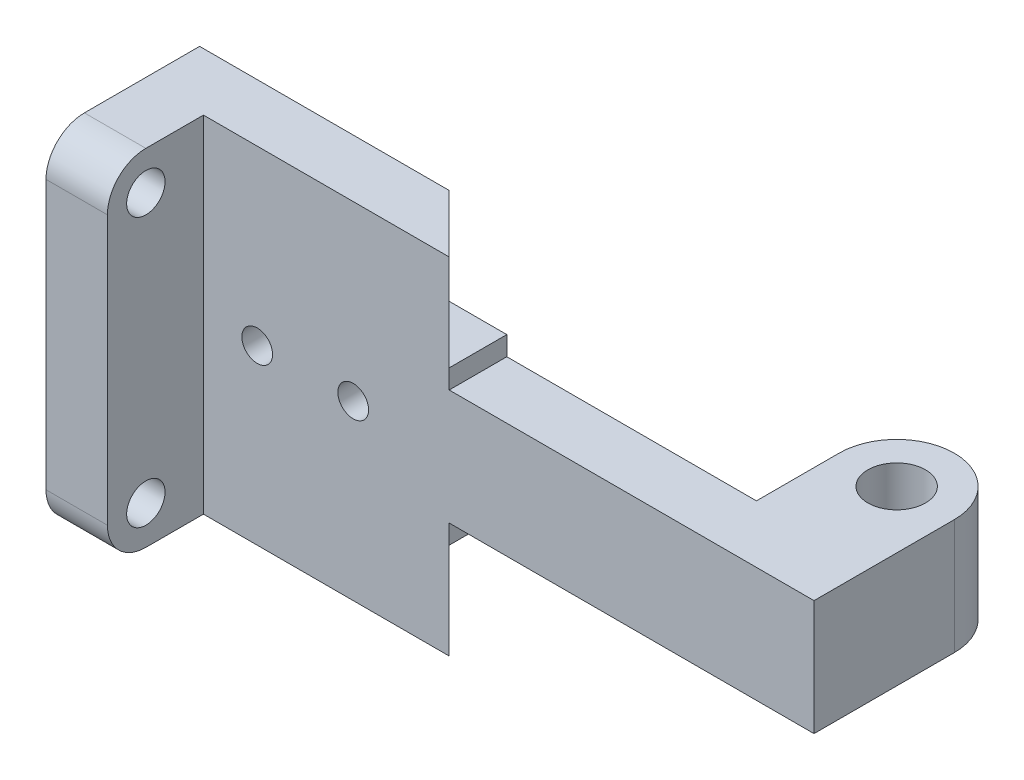
ISO-10303-21;
HEADER;
FILE_DESCRIPTION(('STEP AP214'),'2;1');
FILE_NAME('part.step','',(''),(''),'','','');
FILE_SCHEMA(('AUTOMOTIVE_DESIGN { 1 0 10303 214 1 1 1 1 }'));
ENDSEC;
DATA;
#1=APPLICATION_CONTEXT('core data for automotive mechanical design processes');
#2=APPLICATION_PROTOCOL_DEFINITION('international standard','automotive_design',2000,#1);
#3=PRODUCT_CONTEXT('',#1,'mechanical');
#4=PRODUCT('Part','Part','',(#3));
#5=PRODUCT_RELATED_PRODUCT_CATEGORY('part','',(#4));
#6=PRODUCT_DEFINITION_FORMATION('','',#4);
#7=PRODUCT_DEFINITION_CONTEXT('part definition',#1,'design');
#8=PRODUCT_DEFINITION('design','',#6,#7);
#9=PRODUCT_DEFINITION_SHAPE('','',#8);
#10=(LENGTH_UNIT() NAMED_UNIT(*) SI_UNIT(.MILLI.,.METRE.));
#11=(NAMED_UNIT(*) PLANE_ANGLE_UNIT() SI_UNIT($,.RADIAN.));
#12=(NAMED_UNIT(*) SI_UNIT($,.STERADIAN.) SOLID_ANGLE_UNIT());
#13=UNCERTAINTY_MEASURE_WITH_UNIT(LENGTH_MEASURE(1.E-05),#10,'distance_accuracy_value','');
#14=(GEOMETRIC_REPRESENTATION_CONTEXT(3) GLOBAL_UNCERTAINTY_ASSIGNED_CONTEXT((#13)) GLOBAL_UNIT_ASSIGNED_CONTEXT((#10,
#11,#12)) REPRESENTATION_CONTEXT('',''));
#15=CARTESIAN_POINT('',(0.,0.,0.));
#16=DIRECTION('',(0.,0.,1.));
#17=DIRECTION('',(1.,0.,0.));
#18=AXIS2_PLACEMENT_3D('',#15,#16,#17);
#19=CARTESIAN_POINT('',(-40.,90.,-7.5));
#20=DIRECTION('',(1.,0.,0.));
#21=DIRECTION('',(0.,0.,-1.));
#22=AXIS2_PLACEMENT_3D('',#19,#20,#21);
#23=PLANE('',#22);
#24=DIRECTION('',(0.,0.,1.));
#25=VECTOR('',#24,1.);
#26=CARTESIAN_POINT('',(-40.,0.,-7.5));
#27=LINE('',#26,#25);
#28=CARTESIAN_POINT('',(-40.,0.,-7.5));
#29=VERTEX_POINT('',#28);
#30=CARTESIAN_POINT('',(-40.,0.,22.5));
#31=VERTEX_POINT('',#30);
#32=EDGE_CURVE('E267',#29,#31,#27,.T.);
#33=ORIENTED_EDGE('',*,*,#32,.T.);
#34=CARTESIAN_POINT('',(-40.,9.99999999999999,22.5));
#35=DIRECTION('',(1.,0.,0.));
#36=DIRECTION('',(0.,0.,-1.));
#37=AXIS2_PLACEMENT_3D('',#34,#35,#36);
#38=CIRCLE('',#37,10.);
#39=CARTESIAN_POINT('',(-40.,10.,32.5));
#40=VERTEX_POINT('',#39);
#41=EDGE_CURVE('E48',#31,#40,#38,.F.);
#42=ORIENTED_EDGE('',*,*,#41,.T.);
#43=DIRECTION('',(0.,-1.,0.));
#44=VECTOR('',#43,1.);
#45=CARTESIAN_POINT('',(-40.,90.,32.5));
#46=LINE('',#45,#44);
#47=CARTESIAN_POINT('',(-40.,80.,32.5));
#48=VERTEX_POINT('',#47);
#49=EDGE_CURVE('E279',#48,#40,#46,.T.);
#50=ORIENTED_EDGE('',*,*,#49,.F.);
#51=CARTESIAN_POINT('',(-40.,80.,22.5));
#52=DIRECTION('',(1.,0.,0.));
#53=DIRECTION('',(0.,0.,-1.));
#54=AXIS2_PLACEMENT_3D('',#51,#52,#53);
#55=CIRCLE('',#54,10.);
#56=CARTESIAN_POINT('',(-40.,90.,22.5));
#57=VERTEX_POINT('',#56);
#58=EDGE_CURVE('E57',#48,#57,#55,.F.);
#59=ORIENTED_EDGE('',*,*,#58,.T.);
#60=DIRECTION('',(0.,0.,1.));
#61=VECTOR('',#60,1.);
#62=CARTESIAN_POINT('',(-40.,90.,-7.5));
#63=LINE('',#62,#61);
#64=CARTESIAN_POINT('',(-40.,90.,-7.5));
#65=VERTEX_POINT('',#64);
#66=EDGE_CURVE('E259',#65,#57,#63,.T.);
#67=ORIENTED_EDGE('',*,*,#66,.F.);
#68=DIRECTION('',(0.,-1.,0.));
#69=VECTOR('',#68,1.);
#70=CARTESIAN_POINT('',(-40.,90.,-7.5));
#71=LINE('',#70,#69);
#72=EDGE_CURVE('E283',#65,#29,#71,.T.);
#73=ORIENTED_EDGE('',*,*,#72,.T.);
#74=EDGE_LOOP('',(#33,#42,#50,#59,#67,#73));
#75=FACE_BOUND('',#74,.T.);
#76=CARTESIAN_POINT('',(-40.000012,9.99999999999999,22.5));
#77=DIRECTION('',(-1.,0.,0.));
#78=DIRECTION('',(0.,0.,1.));
#79=AXIS2_PLACEMENT_3D('',#76,#77,#78);
#80=CIRCLE('',#79,5.);
#81=CARTESIAN_POINT('',(-40.000012,9.99999999999999,27.5));
#82=VERTEX_POINT('',#81);
#83=EDGE_CURVE('E309',#82,#82,#80,.T.);
#84=ORIENTED_EDGE('',*,*,#83,.F.);
#85=EDGE_LOOP('',(#84));
#86=FACE_BOUND('',#85,.T.);
#87=CARTESIAN_POINT('',(-40.000012,80.,22.5));
#88=DIRECTION('',(-1.,0.,0.));
#89=DIRECTION('',(0.,0.,1.));
#90=AXIS2_PLACEMENT_3D('',#87,#88,#89);
#91=CIRCLE('',#90,5.);
#92=CARTESIAN_POINT('',(-40.000012,80.,27.5));
#93=VERTEX_POINT('',#92);
#94=EDGE_CURVE('E303',#93,#93,#91,.T.);
#95=ORIENTED_EDGE('',*,*,#94,.F.);
#96=EDGE_LOOP('',(#95));
#97=FACE_BOUND('',#96,.T.);
#98=ADVANCED_FACE('F39',(#75,#86,#97),#23,.F.);
#99=CARTESIAN_POINT('',(40.,90.,-7.5));
#100=DIRECTION('',(-1.,0.,0.));
#101=DIRECTION('',(0.,0.,1.));
#102=AXIS2_PLACEMENT_3D('',#99,#100,#101);
#103=PLANE('',#102);
#104=DIRECTION('',(0.,0.,1.));
#105=VECTOR('',#104,1.);
#106=CARTESIAN_POINT('',(40.,60.,7.5));
#107=LINE('',#106,#105);
#108=CARTESIAN_POINT('',(40.,60.,-7.5));
#109=VERTEX_POINT('',#108);
#110=CARTESIAN_POINT('',(40.,60.,7.5));
#111=VERTEX_POINT('',#110);
#112=EDGE_CURVE('E169',#109,#111,#107,.T.);
#113=ORIENTED_EDGE('',*,*,#112,.F.);
#114=DIRECTION('',(0.,-1.,0.));
#115=VECTOR('',#114,1.);
#116=CARTESIAN_POINT('',(40.,90.,-7.5));
#117=LINE('',#116,#115);
#118=CARTESIAN_POINT('',(40.,65.,-7.5));
#119=VERTEX_POINT('',#118);
#120=EDGE_CURVE('E281',#119,#109,#117,.T.);
#121=ORIENTED_EDGE('',*,*,#120,.F.);
#122=DIRECTION('',(0.,0.,-1.));
#123=VECTOR('',#122,1.);
#124=CARTESIAN_POINT('',(40.,65.,0.));
#125=LINE('',#124,#123);
#126=CARTESIAN_POINT('',(40.,65.,7.5));
#127=VERTEX_POINT('',#126);
#128=EDGE_CURVE('E171',#127,#119,#125,.T.);
#129=ORIENTED_EDGE('',*,*,#128,.F.);
#130=DIRECTION('',(0.,-1.,0.));
#131=VECTOR('',#130,1.);
#132=CARTESIAN_POINT('',(40.,90.,7.5));
#133=LINE('',#132,#131);
#134=EDGE_CURVE('E165',#127,#111,#133,.T.);
#135=ORIENTED_EDGE('',*,*,#134,.T.);
#136=EDGE_LOOP('',(#113,#121,#129,#135));
#137=FACE_BOUND('',#136,.T.);
#138=ADVANCED_FACE('F168',(#137),#103,.F.);
#139=CARTESIAN_POINT('',(40.,30.,-7.5));
#140=VERTEX_POINT('',#139);
#141=CARTESIAN_POINT('',(40.,25.,-7.5));
#142=VERTEX_POINT('',#141);
#143=EDGE_CURVE('E285',#140,#142,#117,.T.);
#144=ORIENTED_EDGE('',*,*,#143,.F.);
#145=DIRECTION('',(0.,0.,1.));
#146=VECTOR('',#145,1.);
#147=CARTESIAN_POINT('',(40.,30.,7.5));
#148=LINE('',#147,#146);
#149=CARTESIAN_POINT('',(40.,30.,7.5));
#150=VERTEX_POINT('',#149);
#151=EDGE_CURVE('E206',#140,#150,#148,.T.);
#152=ORIENTED_EDGE('',*,*,#151,.T.);
#153=CARTESIAN_POINT('',(40.,25.,7.5));
#154=VERTEX_POINT('',#153);
#155=EDGE_CURVE('E174',#150,#154,#133,.T.);
#156=ORIENTED_EDGE('',*,*,#155,.T.);
#157=DIRECTION('',(0.,0.,-1.));
#158=VECTOR('',#157,1.);
#159=CARTESIAN_POINT('',(40.,25.,0.));
#160=LINE('',#159,#158);
#161=EDGE_CURVE('E233',#154,#142,#160,.T.);
#162=ORIENTED_EDGE('',*,*,#161,.T.);
#163=EDGE_LOOP('',(#144,#152,#156,#162));
#164=FACE_BOUND('',#163,.T.);
#165=ADVANCED_FACE('F477',(#164),#103,.F.);
#166=CARTESIAN_POINT('',(-40.,90.,-7.5));
#167=DIRECTION('',(0.,0.,1.));
#168=DIRECTION('',(1.,0.,0.));
#169=AXIS2_PLACEMENT_3D('',#166,#167,#168);
#170=PLANE('',#169);
#171=CARTESIAN_POINT('',(-9.99999999999999,45.,-7.5));
#172=DIRECTION('',(0.,0.,1.));
#173=DIRECTION('',(1.,0.,0.));
#174=AXIS2_PLACEMENT_3D('',#171,#172,#173);
#175=CIRCLE('',#174,4.);
#176=CARTESIAN_POINT('',(-14.,45.,-7.50000000000001));
#177=VERTEX_POINT('',#176);
#178=EDGE_CURVE('E347',#177,#177,#175,.T.);
#179=ORIENTED_EDGE('',*,*,#178,.T.);
#180=EDGE_LOOP('',(#179));
#181=FACE_BOUND('',#180,.T.);
#182=CARTESIAN_POINT('',(15.,45.,-7.5));
#183=DIRECTION('',(0.,0.,1.));
#184=DIRECTION('',(1.,0.,0.));
#185=AXIS2_PLACEMENT_3D('',#182,#183,#184);
#186=CIRCLE('',#185,4.);
#187=CARTESIAN_POINT('',(11.,45.,-7.50000000000001));
#188=VERTEX_POINT('',#187);
#189=EDGE_CURVE('E338',#188,#188,#186,.T.);
#190=ORIENTED_EDGE('',*,*,#189,.T.);
#191=EDGE_LOOP('',(#190));
#192=FACE_BOUND('',#191,.T.);
#193=DIRECTION('',(-1.,0.,0.));
#194=VECTOR('',#193,1.);
#195=CARTESIAN_POINT('',(0.,25.,-7.5));
#196=LINE('',#195,#194);
#197=CARTESIAN_POINT('',(25.0000000000002,25.,-7.5));
#198=VERTEX_POINT('',#197);
#199=EDGE_CURVE('E226',#142,#198,#196,.T.);
#200=ORIENTED_EDGE('',*,*,#199,.T.);
#201=DIRECTION('',(0.,-1.,0.));
#202=VECTOR('',#201,1.);
#203=CARTESIAN_POINT('',(25.0000000000002,25.,-7.5));
#204=LINE('',#203,#202);
#205=CARTESIAN_POINT('',(25.0000000000002,0.,-7.5));
#206=VERTEX_POINT('',#205);
#207=EDGE_CURVE('E239',#198,#206,#204,.T.);
#208=ORIENTED_EDGE('',*,*,#207,.T.);
#209=DIRECTION('',(-1.,0.,0.));
#210=VECTOR('',#209,1.);
#211=CARTESIAN_POINT('',(-40.,0.,-7.5));
#212=LINE('',#211,#210);
#213=EDGE_CURVE('E253',#206,#29,#212,.T.);
#214=ORIENTED_EDGE('',*,*,#213,.T.);
#215=ORIENTED_EDGE('',*,*,#72,.F.);
#216=DIRECTION('',(-1.,0.,0.));
#217=VECTOR('',#216,1.);
#218=CARTESIAN_POINT('',(-24.,90.,-7.5));
#219=LINE('',#218,#217);
#220=CARTESIAN_POINT('',(25.0000000000002,90.,-7.5));
#221=VERTEX_POINT('',#220);
#222=EDGE_CURVE('E257',#221,#65,#219,.T.);
#223=ORIENTED_EDGE('',*,*,#222,.F.);
#224=DIRECTION('',(0.,1.,0.));
#225=VECTOR('',#224,1.);
#226=CARTESIAN_POINT('',(25.0000000000002,65.,-7.5));
#227=LINE('',#226,#225);
#228=CARTESIAN_POINT('',(25.0000000000002,65.,-7.5));
#229=VERTEX_POINT('',#228);
#230=EDGE_CURVE('E255',#229,#221,#227,.T.);
#231=ORIENTED_EDGE('',*,*,#230,.F.);
#232=DIRECTION('',(-1.,0.,0.));
#233=VECTOR('',#232,1.);
#234=CARTESIAN_POINT('',(0.,65.,-7.5));
#235=LINE('',#234,#233);
#236=EDGE_CURVE('E244',#119,#229,#235,.T.);
#237=ORIENTED_EDGE('',*,*,#236,.F.);
#238=ORIENTED_EDGE('',*,*,#120,.T.);
#239=DIRECTION('',(-1.,0.,0.));
#240=VECTOR('',#239,1.);
#241=CARTESIAN_POINT('',(40.,60.,-7.5));
#242=LINE('',#241,#240);
#243=CARTESIAN_POINT('',(105.,60.,-7.5));
#244=VERTEX_POINT('',#243);
#245=EDGE_CURVE('E192',#244,#109,#242,.T.);
#246=ORIENTED_EDGE('',*,*,#245,.F.);
#247=DIRECTION('',(0.,-1.,0.));
#248=VECTOR('',#247,1.);
#249=CARTESIAN_POINT('',(105.,60.,-7.5));
#250=LINE('',#249,#248);
#251=CARTESIAN_POINT('',(105.,30.,-7.5));
#252=VERTEX_POINT('',#251);
#253=EDGE_CURVE('E210',#244,#252,#250,.T.);
#254=ORIENTED_EDGE('',*,*,#253,.T.);
#255=DIRECTION('',(-1.,0.,0.));
#256=VECTOR('',#255,1.);
#257=CARTESIAN_POINT('',(40.,30.,-7.5));
#258=LINE('',#257,#256);
#259=EDGE_CURVE('E195',#252,#140,#258,.T.);
#260=ORIENTED_EDGE('',*,*,#259,.T.);
#261=ORIENTED_EDGE('',*,*,#143,.T.);
#262=EDGE_LOOP('',(#200,#208,#214,#215,#223,#231,#237,#238,#246,#254,#260,#261));
#263=FACE_BOUND('',#262,.T.);
#264=ADVANCED_FACE('F327',(#181,#192,#263),#170,.F.);
#265=CARTESIAN_POINT('',(-40.,90.,32.5));
#266=DIRECTION('',(0.,0.,-1.));
#267=DIRECTION('',(-1.,0.,0.));
#268=AXIS2_PLACEMENT_3D('',#265,#266,#267);
#269=PLANE('',#268);
#270=ORIENTED_EDGE('',*,*,#49,.T.);
#271=DIRECTION('',(1.,0.,0.));
#272=VECTOR('',#271,1.);
#273=CARTESIAN_POINT('',(-40.,9.99999999999999,32.5));
#274=LINE('',#273,#272);
#275=CARTESIAN_POINT('',(-24.,10.,32.5));
#276=VERTEX_POINT('',#275);
#277=EDGE_CURVE('E288',#40,#276,#274,.T.);
#278=ORIENTED_EDGE('',*,*,#277,.T.);
#279=DIRECTION('',(0.,-1.,0.));
#280=VECTOR('',#279,1.);
#281=CARTESIAN_POINT('',(-24.,90.,32.5));
#282=LINE('',#281,#280);
#283=CARTESIAN_POINT('',(-24.,80.,32.5));
#284=VERTEX_POINT('',#283);
#285=EDGE_CURVE('E273',#284,#276,#282,.T.);
#286=ORIENTED_EDGE('',*,*,#285,.F.);
#287=DIRECTION('',(1.,0.,0.));
#288=VECTOR('',#287,1.);
#289=CARTESIAN_POINT('',(-40.,80.,32.5));
#290=LINE('',#289,#288);
#291=EDGE_CURVE('E287',#284,#48,#290,.F.);
#292=ORIENTED_EDGE('',*,*,#291,.T.);
#293=EDGE_LOOP('',(#270,#278,#286,#292));
#294=FACE_BOUND('',#293,.T.);
#295=ADVANCED_FACE('F328',(#294),#269,.F.);
#296=CARTESIAN_POINT('',(-24.,90.,7.5));
#297=DIRECTION('',(-1.,0.,0.));
#298=DIRECTION('',(0.,0.,1.));
#299=AXIS2_PLACEMENT_3D('',#296,#297,#298);
#300=PLANE('',#299);
#301=CARTESIAN_POINT('',(-24.,80.,22.5));
#302=DIRECTION('',(-1.,0.,0.));
#303=DIRECTION('',(0.,0.,1.));
#304=AXIS2_PLACEMENT_3D('',#301,#302,#303);
#305=CIRCLE('',#304,5.);
#306=CARTESIAN_POINT('',(-24.,80.,27.5));
#307=VERTEX_POINT('',#306);
#308=EDGE_CURVE('E305',#307,#307,#305,.T.);
#309=ORIENTED_EDGE('',*,*,#308,.T.);
#310=EDGE_LOOP('',(#309));
#311=FACE_BOUND('',#310,.T.);
#312=CARTESIAN_POINT('',(-24.,9.99999999999999,22.5));
#313=DIRECTION('',(-1.,0.,0.));
#314=DIRECTION('',(0.,0.,1.));
#315=AXIS2_PLACEMENT_3D('',#312,#313,#314);
#316=CIRCLE('',#315,5.);
#317=CARTESIAN_POINT('',(-24.,9.99999999999999,27.5));
#318=VERTEX_POINT('',#317);
#319=EDGE_CURVE('E299',#318,#318,#316,.T.);
#320=ORIENTED_EDGE('',*,*,#319,.T.);
#321=EDGE_LOOP('',(#320));
#322=FACE_BOUND('',#321,.T.);
#323=ORIENTED_EDGE('',*,*,#285,.T.);
#324=CARTESIAN_POINT('',(-24.,9.99999999999999,22.5));
#325=DIRECTION('',(-1.,0.,0.));
#326=DIRECTION('',(0.,0.,1.));
#327=AXIS2_PLACEMENT_3D('',#324,#325,#326);
#328=CIRCLE('',#327,10.);
#329=CARTESIAN_POINT('',(-24.,0.,22.5));
#330=VERTEX_POINT('',#329);
#331=EDGE_CURVE('E295',#276,#330,#328,.F.);
#332=ORIENTED_EDGE('',*,*,#331,.T.);
#333=DIRECTION('',(0.,0.,-1.));
#334=VECTOR('',#333,1.);
#335=CARTESIAN_POINT('',(-24.,0.,7.5));
#336=LINE('',#335,#334);
#337=CARTESIAN_POINT('',(-24.,0.,7.5));
#338=VERTEX_POINT('',#337);
#339=EDGE_CURVE('E268',#330,#338,#336,.T.);
#340=ORIENTED_EDGE('',*,*,#339,.T.);
#341=DIRECTION('',(0.,-1.,0.));
#342=VECTOR('',#341,1.);
#343=CARTESIAN_POINT('',(-24.,90.,7.5));
#344=LINE('',#343,#342);
#345=CARTESIAN_POINT('',(-24.,90.,7.5));
#346=VERTEX_POINT('',#345);
#347=EDGE_CURVE('E275',#346,#338,#344,.T.);
#348=ORIENTED_EDGE('',*,*,#347,.F.);
#349=DIRECTION('',(0.,0.,-1.));
#350=VECTOR('',#349,1.);
#351=CARTESIAN_POINT('',(-24.,90.,7.5));
#352=LINE('',#351,#350);
#353=CARTESIAN_POINT('',(-24.,90.,22.5));
#354=VERTEX_POINT('',#353);
#355=EDGE_CURVE('E263',#354,#346,#352,.T.);
#356=ORIENTED_EDGE('',*,*,#355,.F.);
#357=CARTESIAN_POINT('',(-24.,80.,22.5));
#358=DIRECTION('',(-1.,0.,0.));
#359=DIRECTION('',(0.,0.,1.));
#360=AXIS2_PLACEMENT_3D('',#357,#358,#359);
#361=CIRCLE('',#360,10.);
#362=EDGE_CURVE('E292',#354,#284,#361,.F.);
#363=ORIENTED_EDGE('',*,*,#362,.T.);
#364=EDGE_LOOP('',(#323,#332,#340,#348,#356,#363));
#365=FACE_BOUND('',#364,.T.);
#366=ADVANCED_FACE('F441',(#311,#322,#365),#300,.F.);
#367=CARTESIAN_POINT('',(-24.,90.,7.5));
#368=DIRECTION('',(0.,0.,-1.));
#369=DIRECTION('',(-1.,0.,0.));
#370=AXIS2_PLACEMENT_3D('',#367,#368,#369);
#371=PLANE('',#370);
#372=CARTESIAN_POINT('',(-9.99999999999999,45.,7.5));
#373=DIRECTION('',(0.,0.,-1.));
#374=DIRECTION('',(-1.,0.,0.));
#375=AXIS2_PLACEMENT_3D('',#372,#373,#374);
#376=CIRCLE('',#375,4.);
#377=CARTESIAN_POINT('',(-14.,45.,7.5));
#378=VERTEX_POINT('',#377);
#379=EDGE_CURVE('E43',#378,#378,#376,.T.);
#380=ORIENTED_EDGE('',*,*,#379,.T.);
#381=EDGE_LOOP('',(#380));
#382=FACE_BOUND('',#381,.T.);
#383=CARTESIAN_POINT('',(15.,45.,7.5));
#384=DIRECTION('',(0.,0.,-1.));
#385=DIRECTION('',(-1.,0.,0.));
#386=AXIS2_PLACEMENT_3D('',#383,#384,#385);
#387=CIRCLE('',#386,4.);
#388=CARTESIAN_POINT('',(11.,45.,7.5));
#389=VERTEX_POINT('',#388);
#390=EDGE_CURVE('E334',#389,#389,#387,.T.);
#391=ORIENTED_EDGE('',*,*,#390,.T.);
#392=EDGE_LOOP('',(#391));
#393=FACE_BOUND('',#392,.T.);
#394=DIRECTION('',(1.,0.,0.));
#395=VECTOR('',#394,1.);
#396=CARTESIAN_POINT('',(-24.,0.,7.5));
#397=LINE('',#396,#395);
#398=CARTESIAN_POINT('',(40.,0.,7.5));
#399=VERTEX_POINT('',#398);
#400=EDGE_CURVE('E256',#338,#399,#397,.T.);
#401=ORIENTED_EDGE('',*,*,#400,.T.);
#402=DIRECTION('',(0.,-1.,0.));
#403=VECTOR('',#402,1.);
#404=CARTESIAN_POINT('',(40.,25.,7.5));
#405=LINE('',#404,#403);
#406=EDGE_CURVE('E240',#154,#399,#405,.T.);
#407=ORIENTED_EDGE('',*,*,#406,.F.);
#408=ORIENTED_EDGE('',*,*,#155,.F.);
#409=DIRECTION('',(1.,0.,0.));
#410=VECTOR('',#409,1.);
#411=CARTESIAN_POINT('',(40.,30.,7.5));
#412=LINE('',#411,#410);
#413=CARTESIAN_POINT('',(135.,30.,7.5));
#414=VERTEX_POINT('',#413);
#415=EDGE_CURVE('E208',#150,#414,#412,.T.);
#416=ORIENTED_EDGE('',*,*,#415,.T.);
#417=DIRECTION('',(0.,-1.,0.));
#418=VECTOR('',#417,1.);
#419=CARTESIAN_POINT('',(135.,60.,7.5));
#420=LINE('',#419,#418);
#421=CARTESIAN_POINT('',(135.,60.,7.5));
#422=VERTEX_POINT('',#421);
#423=EDGE_CURVE('E185',#422,#414,#420,.T.);
#424=ORIENTED_EDGE('',*,*,#423,.F.);
#425=DIRECTION('',(1.,0.,0.));
#426=VECTOR('',#425,1.);
#427=CARTESIAN_POINT('',(40.,60.,7.5));
#428=LINE('',#427,#426);
#429=EDGE_CURVE('E178',#111,#422,#428,.T.);
#430=ORIENTED_EDGE('',*,*,#429,.F.);
#431=ORIENTED_EDGE('',*,*,#134,.F.);
#432=CARTESIAN_POINT('',(40.,90.,7.5));
#433=VERTEX_POINT('',#432);
#434=EDGE_CURVE('E172',#433,#127,#133,.T.);
#435=ORIENTED_EDGE('',*,*,#434,.F.);
#436=DIRECTION('',(1.,0.,0.));
#437=VECTOR('',#436,1.);
#438=CARTESIAN_POINT('',(-24.,90.,7.5));
#439=LINE('',#438,#437);
#440=EDGE_CURVE('E262',#346,#433,#439,.T.);
#441=ORIENTED_EDGE('',*,*,#440,.F.);
#442=ORIENTED_EDGE('',*,*,#347,.T.);
#443=EDGE_LOOP('',(#401,#407,#408,#416,#424,#430,#431,#435,#441,#442));
#444=FACE_BOUND('',#443,.T.);
#445=ADVANCED_FACE('F179',(#382,#393,#444),#371,.F.);
#446=CARTESIAN_POINT('',(0.,90.,0.));
#447=DIRECTION('',(0.,1.,0.));
#448=DIRECTION('',(0.,0.,1.));
#449=AXIS2_PLACEMENT_3D('',#446,#447,#448);
#450=PLANE('',#449);
#451=ORIENTED_EDGE('',*,*,#66,.T.);
#452=DIRECTION('',(1.,0.,0.));
#453=VECTOR('',#452,1.);
#454=CARTESIAN_POINT('',(-24.,90.,22.5));
#455=LINE('',#454,#453);
#456=EDGE_CURVE('E11',#57,#354,#455,.T.);
#457=ORIENTED_EDGE('',*,*,#456,.T.);
#458=ORIENTED_EDGE('',*,*,#355,.T.);
#459=ORIENTED_EDGE('',*,*,#440,.T.);
#460=DIRECTION('',(0.707106781186544,0.,0.707106781186551));
#461=VECTOR('',#460,1.);
#462=CARTESIAN_POINT('',(16.2500000000002,90.,-16.25));
#463=LINE('',#462,#461);
#464=EDGE_CURVE('E243',#221,#433,#463,.T.);
#465=ORIENTED_EDGE('',*,*,#464,.F.);
#466=ORIENTED_EDGE('',*,*,#222,.T.);
#467=EDGE_LOOP('',(#451,#457,#458,#459,#465,#466));
#468=FACE_BOUND('',#467,.T.);
#469=ADVANCED_FACE('F432',(#468),#450,.T.);
#470=CARTESIAN_POINT('',(0.,0.,0.));
#471=DIRECTION('',(0.,1.,0.));
#472=DIRECTION('',(0.,0.,1.));
#473=AXIS2_PLACEMENT_3D('',#470,#471,#472);
#474=PLANE('',#473);
#475=ORIENTED_EDGE('',*,*,#339,.F.);
#476=DIRECTION('',(1.,0.,0.));
#477=VECTOR('',#476,1.);
#478=CARTESIAN_POINT('',(0.,0.,22.5));
#479=LINE('',#478,#477);
#480=EDGE_CURVE('E61',#330,#31,#479,.F.);
#481=ORIENTED_EDGE('',*,*,#480,.T.);
#482=ORIENTED_EDGE('',*,*,#32,.F.);
#483=ORIENTED_EDGE('',*,*,#213,.F.);
#484=DIRECTION('',(0.707106781186544,0.,0.707106781186551));
#485=VECTOR('',#484,1.);
#486=CARTESIAN_POINT('',(16.2500000000002,0.,-16.25));
#487=LINE('',#486,#485);
#488=EDGE_CURVE('E227',#206,#399,#487,.T.);
#489=ORIENTED_EDGE('',*,*,#488,.T.);
#490=ORIENTED_EDGE('',*,*,#400,.F.);
#491=EDGE_LOOP('',(#475,#481,#482,#483,#489,#490));
#492=FACE_BOUND('',#491,.T.);
#493=ADVANCED_FACE('F435',(#492),#474,.F.);
#494=CARTESIAN_POINT('',(16.2500000000002,65.,-16.25));
#495=DIRECTION('',(-0.707106781186551,0.,0.707106781186544));
#496=DIRECTION('',(0.707106781186544,0.,0.707106781186551));
#497=AXIS2_PLACEMENT_3D('',#494,#495,#496);
#498=PLANE('',#497);
#499=ORIENTED_EDGE('',*,*,#464,.T.);
#500=ORIENTED_EDGE('',*,*,#434,.T.);
#501=DIRECTION('',(0.707106781186544,0.,0.707106781186551));
#502=VECTOR('',#501,1.);
#503=CARTESIAN_POINT('',(16.2500000000002,65.,-16.25));
#504=LINE('',#503,#502);
#505=EDGE_CURVE('E247',#229,#127,#504,.T.);
#506=ORIENTED_EDGE('',*,*,#505,.F.);
#507=ORIENTED_EDGE('',*,*,#230,.T.);
#508=EDGE_LOOP('',(#499,#500,#506,#507));
#509=FACE_BOUND('',#508,.T.);
#510=ADVANCED_FACE('F426',(#509),#498,.F.);
#511=CARTESIAN_POINT('',(0.,65.,0.));
#512=DIRECTION('',(0.,1.,0.));
#513=DIRECTION('',(0.,0.,1.));
#514=AXIS2_PLACEMENT_3D('',#511,#512,#513);
#515=PLANE('',#514);
#516=ORIENTED_EDGE('',*,*,#236,.T.);
#517=ORIENTED_EDGE('',*,*,#505,.T.);
#518=ORIENTED_EDGE('',*,*,#128,.T.);
#519=EDGE_LOOP('',(#516,#517,#518));
#520=FACE_BOUND('',#519,.T.);
#521=ADVANCED_FACE('F425',(#520),#515,.T.);
#522=CARTESIAN_POINT('',(16.2500000000002,25.,-16.25));
#523=DIRECTION('',(0.707106781186551,0.,-0.707106781186544));
#524=DIRECTION('',(-0.707106781186544,0.,-0.707106781186551));
#525=AXIS2_PLACEMENT_3D('',#522,#523,#524);
#526=PLANE('',#525);
#527=ORIENTED_EDGE('',*,*,#488,.F.);
#528=ORIENTED_EDGE('',*,*,#207,.F.);
#529=DIRECTION('',(0.707106781186544,0.,0.707106781186551));
#530=VECTOR('',#529,1.);
#531=CARTESIAN_POINT('',(16.2500000000002,25.,-16.25));
#532=LINE('',#531,#530);
#533=EDGE_CURVE('E234',#198,#154,#532,.T.);
#534=ORIENTED_EDGE('',*,*,#533,.T.);
#535=ORIENTED_EDGE('',*,*,#406,.T.);
#536=EDGE_LOOP('',(#527,#528,#534,#535));
#537=FACE_BOUND('',#536,.T.);
#538=ADVANCED_FACE('F420',(#537),#526,.T.);
#539=CARTESIAN_POINT('',(0.,25.,0.));
#540=DIRECTION('',(0.,-1.,0.));
#541=DIRECTION('',(0.,0.,1.));
#542=AXIS2_PLACEMENT_3D('',#539,#540,#541);
#543=PLANE('',#542);
#544=ORIENTED_EDGE('',*,*,#199,.F.);
#545=ORIENTED_EDGE('',*,*,#161,.F.);
#546=ORIENTED_EDGE('',*,*,#533,.F.);
#547=EDGE_LOOP('',(#544,#545,#546));
#548=FACE_BOUND('',#547,.T.);
#549=ADVANCED_FACE('F417',(#548),#543,.T.);
#550=CARTESIAN_POINT('',(120.,60.,-29.0249056277761));
#551=DIRECTION('',(0.,1.,0.));
#552=DIRECTION('',(0.,0.,1.));
#553=AXIS2_PLACEMENT_3D('',#550,#551,#552);
#554=PLANE('',#553);
#555=ORIENTED_EDGE('',*,*,#112,.T.);
#556=ORIENTED_EDGE('',*,*,#429,.T.);
#557=DIRECTION('',(0.,0.,-1.));
#558=VECTOR('',#557,1.);
#559=CARTESIAN_POINT('',(135.,60.,-29.0249056277761));
#560=LINE('',#559,#558);
#561=CARTESIAN_POINT('',(135.,60.,-29.0249056277761));
#562=VERTEX_POINT('',#561);
#563=EDGE_CURVE('E184',#422,#562,#560,.T.);
#564=ORIENTED_EDGE('',*,*,#563,.T.);
#565=CARTESIAN_POINT('',(120.,60.,-29.0249056277761));
#566=DIRECTION('',(0.,1.,0.));
#567=DIRECTION('',(0.,0.,1.));
#568=AXIS2_PLACEMENT_3D('',#565,#566,#567);
#569=CIRCLE('',#568,15.);
#570=CARTESIAN_POINT('',(105.,60.,-29.0249056277761));
#571=VERTEX_POINT('',#570);
#572=EDGE_CURVE('E202',#562,#571,#569,.T.);
#573=ORIENTED_EDGE('',*,*,#572,.T.);
#574=DIRECTION('',(0.,0.,1.));
#575=VECTOR('',#574,1.);
#576=CARTESIAN_POINT('',(105.,60.,-29.0249056277761));
#577=LINE('',#576,#575);
#578=EDGE_CURVE('E203',#571,#244,#577,.T.);
#579=ORIENTED_EDGE('',*,*,#578,.T.);
#580=ORIENTED_EDGE('',*,*,#245,.T.);
#581=EDGE_LOOP('',(#555,#556,#564,#573,#579,#580));
#582=FACE_BOUND('',#581,.T.);
#583=CARTESIAN_POINT('',(120.,60.,-29.0249056277761));
#584=DIRECTION('',(0.,1.,0.));
#585=DIRECTION('',(0.,0.,1.));
#586=AXIS2_PLACEMENT_3D('',#583,#584,#585);
#587=CIRCLE('',#586,7.50000000000003);
#588=CARTESIAN_POINT('',(120.,60.,-21.5249056277761));
#589=VERTEX_POINT('',#588);
#590=EDGE_CURVE('E212',#589,#589,#587,.T.);
#591=ORIENTED_EDGE('',*,*,#590,.F.);
#592=EDGE_LOOP('',(#591));
#593=FACE_BOUND('',#592,.T.);
#594=ADVANCED_FACE('F189',(#582,#593),#554,.T.);
#595=CARTESIAN_POINT('',(120.,30.,-29.0249056277761));
#596=DIRECTION('',(0.,1.,0.));
#597=DIRECTION('',(0.,0.,1.));
#598=AXIS2_PLACEMENT_3D('',#595,#596,#597);
#599=PLANE('',#598);
#600=ORIENTED_EDGE('',*,*,#151,.F.);
#601=ORIENTED_EDGE('',*,*,#259,.F.);
#602=DIRECTION('',(0.,0.,1.));
#603=VECTOR('',#602,1.);
#604=CARTESIAN_POINT('',(105.,30.,-29.0249056277761));
#605=LINE('',#604,#603);
#606=CARTESIAN_POINT('',(105.,30.,-29.0249056277761));
#607=VERTEX_POINT('',#606);
#608=EDGE_CURVE('E193',#607,#252,#605,.T.);
#609=ORIENTED_EDGE('',*,*,#608,.F.);
#610=CARTESIAN_POINT('',(120.,30.,-29.0249056277761));
#611=DIRECTION('',(0.,1.,0.));
#612=DIRECTION('',(0.,0.,1.));
#613=AXIS2_PLACEMENT_3D('',#610,#611,#612);
#614=CIRCLE('',#613,15.);
#615=CARTESIAN_POINT('',(135.,30.,-29.0249056277761));
#616=VERTEX_POINT('',#615);
#617=EDGE_CURVE('E213',#616,#607,#614,.T.);
#618=ORIENTED_EDGE('',*,*,#617,.F.);
#619=DIRECTION('',(0.,0.,-1.));
#620=VECTOR('',#619,1.);
#621=CARTESIAN_POINT('',(135.,30.,-29.0249056277761));
#622=LINE('',#621,#620);
#623=EDGE_CURVE('E214',#414,#616,#622,.T.);
#624=ORIENTED_EDGE('',*,*,#623,.F.);
#625=ORIENTED_EDGE('',*,*,#415,.F.);
#626=EDGE_LOOP('',(#600,#601,#609,#618,#624,#625));
#627=FACE_BOUND('',#626,.T.);
#628=CARTESIAN_POINT('',(120.,30.,-29.0249056277761));
#629=DIRECTION('',(0.,1.,0.));
#630=DIRECTION('',(0.,0.,1.));
#631=AXIS2_PLACEMENT_3D('',#628,#629,#630);
#632=CIRCLE('',#631,7.50000000000003);
#633=CARTESIAN_POINT('',(120.,30.,-21.5249056277761));
#634=VERTEX_POINT('',#633);
#635=EDGE_CURVE('E197',#634,#634,#632,.T.);
#636=ORIENTED_EDGE('',*,*,#635,.T.);
#637=EDGE_LOOP('',(#636));
#638=FACE_BOUND('',#637,.T.);
#639=ADVANCED_FACE('F394',(#627,#638),#599,.F.);
#640=CARTESIAN_POINT('',(135.,60.,-29.0249056277761));
#641=DIRECTION('',(-1.,0.,0.));
#642=DIRECTION('',(0.,0.,1.));
#643=AXIS2_PLACEMENT_3D('',#640,#641,#642);
#644=PLANE('',#643);
#645=ORIENTED_EDGE('',*,*,#623,.T.);
#646=DIRECTION('',(0.,-1.,0.));
#647=VECTOR('',#646,1.);
#648=CARTESIAN_POINT('',(135.,60.,-29.0249056277761));
#649=LINE('',#648,#647);
#650=EDGE_CURVE('E224',#562,#616,#649,.T.);
#651=ORIENTED_EDGE('',*,*,#650,.F.);
#652=ORIENTED_EDGE('',*,*,#563,.F.);
#653=ORIENTED_EDGE('',*,*,#423,.T.);
#654=EDGE_LOOP('',(#645,#651,#652,#653));
#655=FACE_BOUND('',#654,.T.);
#656=ADVANCED_FACE('F406',(#655),#644,.F.);
#657=CARTESIAN_POINT('',(120.,60.,-29.0249056277761));
#658=DIRECTION('',(0.,-1.,0.));
#659=DIRECTION('',(0.,0.,-1.));
#660=AXIS2_PLACEMENT_3D('',#657,#658,#659);
#661=CYLINDRICAL_SURFACE('',#660,15.);
#662=ORIENTED_EDGE('',*,*,#617,.T.);
#663=DIRECTION('',(0.,-1.,0.));
#664=VECTOR('',#663,1.);
#665=CARTESIAN_POINT('',(105.,60.,-29.0249056277761));
#666=LINE('',#665,#664);
#667=EDGE_CURVE('E216',#571,#607,#666,.T.);
#668=ORIENTED_EDGE('',*,*,#667,.F.);
#669=ORIENTED_EDGE('',*,*,#572,.F.);
#670=ORIENTED_EDGE('',*,*,#650,.T.);
#671=EDGE_LOOP('',(#662,#668,#669,#670));
#672=FACE_BOUND('',#671,.T.);
#673=ADVANCED_FACE('F401',(#672),#661,.T.);
#674=CARTESIAN_POINT('',(105.,60.,-29.0249056277761));
#675=DIRECTION('',(1.,0.,0.));
#676=DIRECTION('',(0.,0.,-1.));
#677=AXIS2_PLACEMENT_3D('',#674,#675,#676);
#678=PLANE('',#677);
#679=ORIENTED_EDGE('',*,*,#608,.T.);
#680=ORIENTED_EDGE('',*,*,#253,.F.);
#681=ORIENTED_EDGE('',*,*,#578,.F.);
#682=ORIENTED_EDGE('',*,*,#667,.T.);
#683=EDGE_LOOP('',(#679,#680,#681,#682));
#684=FACE_BOUND('',#683,.T.);
#685=ADVANCED_FACE('F396',(#684),#678,.F.);
#686=CARTESIAN_POINT('',(120.,60.,-29.0249056277761));
#687=DIRECTION('',(0.,-1.,0.));
#688=DIRECTION('',(0.,0.,-1.));
#689=AXIS2_PLACEMENT_3D('',#686,#687,#688);
#690=CYLINDRICAL_SURFACE('',#689,7.50000000000003);
#691=ORIENTED_EDGE('',*,*,#590,.T.);
#692=EDGE_LOOP('',(#691));
#693=FACE_BOUND('',#692,.T.);
#694=ORIENTED_EDGE('',*,*,#635,.F.);
#695=EDGE_LOOP('',(#694));
#696=FACE_BOUND('',#695,.T.);
#697=ADVANCED_FACE('F380',(#693,#696),#690,.F.);
#698=CARTESIAN_POINT('',(-40.,9.99999999999999,22.5));
#699=DIRECTION('',(1.,0.,0.));
#700=DIRECTION('',(0.,0.,-1.));
#701=AXIS2_PLACEMENT_3D('',#698,#699,#700);
#702=CYLINDRICAL_SURFACE('',#701,10.);
#703=ORIENTED_EDGE('',*,*,#41,.F.);
#704=ORIENTED_EDGE('',*,*,#480,.F.);
#705=ORIENTED_EDGE('',*,*,#331,.F.);
#706=ORIENTED_EDGE('',*,*,#277,.F.);
#707=EDGE_LOOP('',(#703,#704,#705,#706));
#708=FACE_BOUND('',#707,.T.);
#709=ADVANCED_FACE('F391',(#708),#702,.T.);
#710=CARTESIAN_POINT('',(0.,80.,22.5));
#711=DIRECTION('',(-1.,0.,0.));
#712=DIRECTION('',(0.,0.,1.));
#713=AXIS2_PLACEMENT_3D('',#710,#711,#712);
#714=CYLINDRICAL_SURFACE('',#713,10.);
#715=ORIENTED_EDGE('',*,*,#58,.F.);
#716=ORIENTED_EDGE('',*,*,#291,.F.);
#717=ORIENTED_EDGE('',*,*,#362,.F.);
#718=ORIENTED_EDGE('',*,*,#456,.F.);
#719=EDGE_LOOP('',(#715,#716,#717,#718));
#720=FACE_BOUND('',#719,.T.);
#721=ADVANCED_FACE('F41',(#720),#714,.T.);
#722=CARTESIAN_POINT('',(135.,9.99999999999999,22.5));
#723=DIRECTION('',(-1.,0.,0.));
#724=DIRECTION('',(0.,0.,1.));
#725=AXIS2_PLACEMENT_3D('',#722,#723,#724);
#726=CYLINDRICAL_SURFACE('',#725,5.);
#727=ORIENTED_EDGE('',*,*,#83,.T.);
#728=EDGE_LOOP('',(#727));
#729=FACE_BOUND('',#728,.T.);
#730=ORIENTED_EDGE('',*,*,#319,.F.);
#731=EDGE_LOOP('',(#730));
#732=FACE_BOUND('',#731,.T.);
#733=ADVANCED_FACE('F371',(#729,#732),#726,.F.);
#734=CARTESIAN_POINT('',(135.,80.,22.5));
#735=DIRECTION('',(-1.,0.,0.));
#736=DIRECTION('',(0.,0.,1.));
#737=AXIS2_PLACEMENT_3D('',#734,#735,#736);
#738=CYLINDRICAL_SURFACE('',#737,5.);
#739=ORIENTED_EDGE('',*,*,#94,.T.);
#740=EDGE_LOOP('',(#739));
#741=FACE_BOUND('',#740,.T.);
#742=ORIENTED_EDGE('',*,*,#308,.F.);
#743=EDGE_LOOP('',(#742));
#744=FACE_BOUND('',#743,.T.);
#745=ADVANCED_FACE('F359',(#741,#744),#738,.F.);
#746=CARTESIAN_POINT('',(15.,45.,32.5));
#747=DIRECTION('',(0.,0.,-1.));
#748=DIRECTION('',(-1.,0.,0.));
#749=AXIS2_PLACEMENT_3D('',#746,#747,#748);
#750=CYLINDRICAL_SURFACE('',#749,4.);
#751=CARTESIAN_POINT('',(11.,45.,7.5));
#752=CARTESIAN_POINT('',(11.,45.,7.34375));
#753=CARTESIAN_POINT('',(11.,45.,7.1875));
#754=CARTESIAN_POINT('',(11.,45.,6.875));
#755=CARTESIAN_POINT('',(11.,45.,6.71875));
#756=CARTESIAN_POINT('',(11.,45.,6.40625));
#757=CARTESIAN_POINT('',(11.,45.,6.25));
#758=CARTESIAN_POINT('',(11.,45.,5.9375));
#759=CARTESIAN_POINT('',(11.,45.,5.78125));
#760=CARTESIAN_POINT('',(11.,45.,5.46875));
#761=CARTESIAN_POINT('',(11.,45.,5.3125));
#762=CARTESIAN_POINT('',(11.,45.,5.));
#763=CARTESIAN_POINT('',(11.,45.,4.84375));
#764=CARTESIAN_POINT('',(11.,45.,4.53125));
#765=CARTESIAN_POINT('',(11.,45.,4.375));
#766=CARTESIAN_POINT('',(11.,45.,4.0625));
#767=CARTESIAN_POINT('',(11.,45.,3.90625));
#768=CARTESIAN_POINT('',(11.,45.,3.59375));
#769=CARTESIAN_POINT('',(11.,45.,3.4375));
#770=CARTESIAN_POINT('',(11.,45.,3.125));
#771=CARTESIAN_POINT('',(11.,45.,2.96875));
#772=CARTESIAN_POINT('',(11.,45.,2.65625));
#773=CARTESIAN_POINT('',(11.,45.,2.5));
#774=CARTESIAN_POINT('',(11.,45.,2.1875));
#775=CARTESIAN_POINT('',(11.,45.,2.03125));
#776=CARTESIAN_POINT('',(11.,45.,1.71875));
#777=CARTESIAN_POINT('',(11.,45.,1.5625));
#778=CARTESIAN_POINT('',(11.,45.,1.25));
#779=CARTESIAN_POINT('',(11.,45.,1.09375));
#780=CARTESIAN_POINT('',(11.,45.,0.781249999999995));
#781=CARTESIAN_POINT('',(11.,45.,0.624999999999996));
#782=CARTESIAN_POINT('',(11.,45.,0.312499999999998));
#783=CARTESIAN_POINT('',(11.,45.,0.156249999999999));
#784=CARTESIAN_POINT('',(11.,45.,-0.156250000000001));
#785=CARTESIAN_POINT('',(11.,45.,-0.312500000000003));
#786=CARTESIAN_POINT('',(11.,45.,-0.625000000000005));
#787=CARTESIAN_POINT('',(11.,45.,-0.781250000000006));
#788=CARTESIAN_POINT('',(11.,45.,-1.09375000000001));
#789=CARTESIAN_POINT('',(11.,45.,-1.25000000000001));
#790=CARTESIAN_POINT('',(11.,45.,-1.5625));
#791=CARTESIAN_POINT('',(11.,45.,-1.71875));
#792=CARTESIAN_POINT('',(11.,45.,-2.03125));
#793=CARTESIAN_POINT('',(11.,45.,-2.1875));
#794=CARTESIAN_POINT('',(11.,45.,-2.5));
#795=CARTESIAN_POINT('',(11.,45.,-2.65625));
#796=CARTESIAN_POINT('',(11.,45.,-2.96875));
#797=CARTESIAN_POINT('',(11.,45.,-3.125));
#798=CARTESIAN_POINT('',(11.,45.,-3.43750000000001));
#799=CARTESIAN_POINT('',(11.,45.,-3.59375));
#800=CARTESIAN_POINT('',(11.,45.,-3.90625));
#801=CARTESIAN_POINT('',(11.,45.,-4.06250000000001));
#802=CARTESIAN_POINT('',(11.,45.,-4.37500000000001));
#803=CARTESIAN_POINT('',(11.,45.,-4.53125000000001));
#804=CARTESIAN_POINT('',(11.,45.,-4.84375000000001));
#805=CARTESIAN_POINT('',(11.,45.,-5.00000000000001));
#806=CARTESIAN_POINT('',(11.,45.,-5.31250000000001));
#807=CARTESIAN_POINT('',(11.,45.,-5.46875000000001));
#808=CARTESIAN_POINT('',(11.,45.,-5.78125000000001));
#809=CARTESIAN_POINT('',(11.,45.,-5.93750000000001));
#810=CARTESIAN_POINT('',(11.,45.,-6.25000000000001));
#811=CARTESIAN_POINT('',(11.,45.,-6.40625000000001));
#812=CARTESIAN_POINT('',(11.,45.,-6.71875000000001));
#813=CARTESIAN_POINT('',(11.,45.,-6.875));
#814=CARTESIAN_POINT('',(11.,45.,-7.1875));
#815=CARTESIAN_POINT('',(11.,45.,-7.34375));
#816=CARTESIAN_POINT('',(11.,45.,-7.50000000000001));
#817=B_SPLINE_CURVE_WITH_KNOTS('',3,(#751,#752,#753,#754,#755,#756,#757,#758,#759,#760,#761,
#762,#763,#764,#765,#766,#767,#768,#769,#770,#771,#772,#773,#774,#775,#776,#777,#778,#779,#780,
#781,#782,#783,#784,#785,#786,#787,#788,#789,#790,#791,#792,#793,#794,#795,#796,#797,#798,#799,
#800,#801,#802,#803,#804,#805,#806,#807,#808,#809,#810,#811,#812,#813,#814,#815,#816),
.UNSPECIFIED.,.F.,.F.,(4,2,2,2,2,2,2,2,2,2,2,2,2,2,2,2,2,2,2,2,2,2,2,2,2,2,2,2,2,2,2,2,4),(0.,
0.46875,0.937500000000001,1.40625,1.875,2.34375,2.8125,3.28125,3.75,4.21875,4.6875,5.15625,
5.625,6.09375,6.56250000000001,7.03125,7.5,7.96875,8.43750000000001,8.90625,9.375,
9.84375000000001,10.3125,10.78125,11.25,11.71875,12.1875,12.65625,13.125,13.59375,14.0625,
14.53125,15.),.UNSPECIFIED.);
#818=EDGE_CURVE('BSEAM369',#389,#188,#817,.T.);
#819=ORIENTED_EDGE('',*,*,#390,.F.);
#820=ORIENTED_EDGE('',*,*,#189,.F.);
#821=ORIENTED_EDGE('',*,*,#818,.T.);
#822=ORIENTED_EDGE('',*,*,#818,.F.);
#823=EDGE_LOOP('',(#819,#821,#820,#822));
#824=FACE_BOUND('',#823,.T.);
#825=ADVANCED_FACE('F369',(#824),#750,.F.);
#826=CARTESIAN_POINT('',(-9.99999999999999,45.,32.5));
#827=DIRECTION('',(0.,0.,-1.));
#828=DIRECTION('',(-1.,0.,0.));
#829=AXIS2_PLACEMENT_3D('',#826,#827,#828);
#830=CYLINDRICAL_SURFACE('',#829,4.);
#831=CARTESIAN_POINT('',(-14.,45.,7.5));
#832=CARTESIAN_POINT('',(-14.,45.,7.34375));
#833=CARTESIAN_POINT('',(-14.,45.,7.1875));
#834=CARTESIAN_POINT('',(-14.,45.,6.875));
#835=CARTESIAN_POINT('',(-14.,45.,6.71875));
#836=CARTESIAN_POINT('',(-14.,45.,6.40625));
#837=CARTESIAN_POINT('',(-14.,45.,6.25));
#838=CARTESIAN_POINT('',(-14.,45.,5.9375));
#839=CARTESIAN_POINT('',(-14.,45.,5.78125));
#840=CARTESIAN_POINT('',(-14.,45.,5.46875));
#841=CARTESIAN_POINT('',(-14.,45.,5.3125));
#842=CARTESIAN_POINT('',(-14.,45.,5.));
#843=CARTESIAN_POINT('',(-14.,45.,4.84375));
#844=CARTESIAN_POINT('',(-14.,45.,4.53125));
#845=CARTESIAN_POINT('',(-14.,45.,4.375));
#846=CARTESIAN_POINT('',(-14.,45.,4.0625));
#847=CARTESIAN_POINT('',(-14.,45.,3.90625));
#848=CARTESIAN_POINT('',(-14.,45.,3.59375));
#849=CARTESIAN_POINT('',(-14.,45.,3.4375));
#850=CARTESIAN_POINT('',(-14.,45.,3.125));
#851=CARTESIAN_POINT('',(-14.,45.,2.96875));
#852=CARTESIAN_POINT('',(-14.,45.,2.65625));
#853=CARTESIAN_POINT('',(-14.,45.,2.5));
#854=CARTESIAN_POINT('',(-14.,45.,2.1875));
#855=CARTESIAN_POINT('',(-14.,45.,2.03125));
#856=CARTESIAN_POINT('',(-14.,45.,1.71875));
#857=CARTESIAN_POINT('',(-14.,45.,1.5625));
#858=CARTESIAN_POINT('',(-14.,45.,1.25));
#859=CARTESIAN_POINT('',(-14.,45.,1.09375));
#860=CARTESIAN_POINT('',(-14.,45.,0.781249999999995));
#861=CARTESIAN_POINT('',(-14.,45.,0.624999999999996));
#862=CARTESIAN_POINT('',(-14.,45.,0.312499999999998));
#863=CARTESIAN_POINT('',(-14.,45.,0.156249999999999));
#864=CARTESIAN_POINT('',(-14.,45.,-0.156250000000001));
#865=CARTESIAN_POINT('',(-14.,45.,-0.312500000000003));
#866=CARTESIAN_POINT('',(-14.,45.,-0.625000000000005));
#867=CARTESIAN_POINT('',(-14.,45.,-0.781250000000006));
#868=CARTESIAN_POINT('',(-14.,45.,-1.09375000000001));
#869=CARTESIAN_POINT('',(-14.,45.,-1.25000000000001));
#870=CARTESIAN_POINT('',(-14.,45.,-1.5625));
#871=CARTESIAN_POINT('',(-14.,45.,-1.71875));
#872=CARTESIAN_POINT('',(-14.,45.,-2.03125));
#873=CARTESIAN_POINT('',(-14.,45.,-2.1875));
#874=CARTESIAN_POINT('',(-14.,45.,-2.5));
#875=CARTESIAN_POINT('',(-14.,45.,-2.65625));
#876=CARTESIAN_POINT('',(-14.,45.,-2.96875));
#877=CARTESIAN_POINT('',(-14.,45.,-3.125));
#878=CARTESIAN_POINT('',(-14.,45.,-3.43750000000001));
#879=CARTESIAN_POINT('',(-14.,45.,-3.59375));
#880=CARTESIAN_POINT('',(-14.,45.,-3.90625));
#881=CARTESIAN_POINT('',(-14.,45.,-4.06250000000001));
#882=CARTESIAN_POINT('',(-14.,45.,-4.37500000000001));
#883=CARTESIAN_POINT('',(-14.,45.,-4.53125000000001));
#884=CARTESIAN_POINT('',(-14.,45.,-4.84375000000001));
#885=CARTESIAN_POINT('',(-14.,45.,-5.00000000000001));
#886=CARTESIAN_POINT('',(-14.,45.,-5.31250000000001));
#887=CARTESIAN_POINT('',(-14.,45.,-5.46875000000001));
#888=CARTESIAN_POINT('',(-14.,45.,-5.78125000000001));
#889=CARTESIAN_POINT('',(-14.,45.,-5.93750000000001));
#890=CARTESIAN_POINT('',(-14.,45.,-6.25000000000001));
#891=CARTESIAN_POINT('',(-14.,45.,-6.40625000000001));
#892=CARTESIAN_POINT('',(-14.,45.,-6.71875000000001));
#893=CARTESIAN_POINT('',(-14.,45.,-6.875));
#894=CARTESIAN_POINT('',(-14.,45.,-7.1875));
#895=CARTESIAN_POINT('',(-14.,45.,-7.34375));
#896=CARTESIAN_POINT('',(-14.,45.,-7.50000000000001));
#897=B_SPLINE_CURVE_WITH_KNOTS('',3,(#831,#832,#833,#834,#835,#836,#837,#838,#839,#840,#841,
#842,#843,#844,#845,#846,#847,#848,#849,#850,#851,#852,#853,#854,#855,#856,#857,#858,#859,#860,
#861,#862,#863,#864,#865,#866,#867,#868,#869,#870,#871,#872,#873,#874,#875,#876,#877,#878,#879,
#880,#881,#882,#883,#884,#885,#886,#887,#888,#889,#890,#891,#892,#893,#894,#895,#896),
.UNSPECIFIED.,.F.,.F.,(4,2,2,2,2,2,2,2,2,2,2,2,2,2,2,2,2,2,2,2,2,2,2,2,2,2,2,2,2,2,2,2,4),(0.,
0.46875,0.937500000000001,1.40625,1.875,2.34375,2.8125,3.28125,3.75,4.21875,4.6875,5.15625,
5.625,6.09375,6.56250000000001,7.03125,7.5,7.96875,8.43750000000001,8.90625,9.375,
9.84375000000001,10.3125,10.78125,11.25,11.71875,12.1875,12.65625,13.125,13.59375,14.0625,
14.53125,15.),.UNSPECIFIED.);
#898=EDGE_CURVE('BSEAM610',#378,#177,#897,.T.);
#899=ORIENTED_EDGE('',*,*,#379,.F.);
#900=ORIENTED_EDGE('',*,*,#178,.F.);
#901=ORIENTED_EDGE('',*,*,#898,.T.);
#902=ORIENTED_EDGE('',*,*,#898,.F.);
#903=EDGE_LOOP('',(#899,#901,#900,#902));
#904=FACE_BOUND('',#903,.T.);
#905=ADVANCED_FACE('F610',(#904),#830,.F.);
#906=CLOSED_SHELL('',(#98,#138,#165,#264,#295,#366,#445,#469,#493,#510,#521,#538,#549,#594,#639,
#656,#673,#685,#697,#709,#721,#733,#745,#825,#905));
#907=MANIFOLD_SOLID_BREP('B2',#906);
#908=ADVANCED_BREP_SHAPE_REPRESENTATION('',(#18,#907),#14);
#909=SHAPE_DEFINITION_REPRESENTATION(#9,#908);
ENDSEC;
END-ISO-10303-21;
